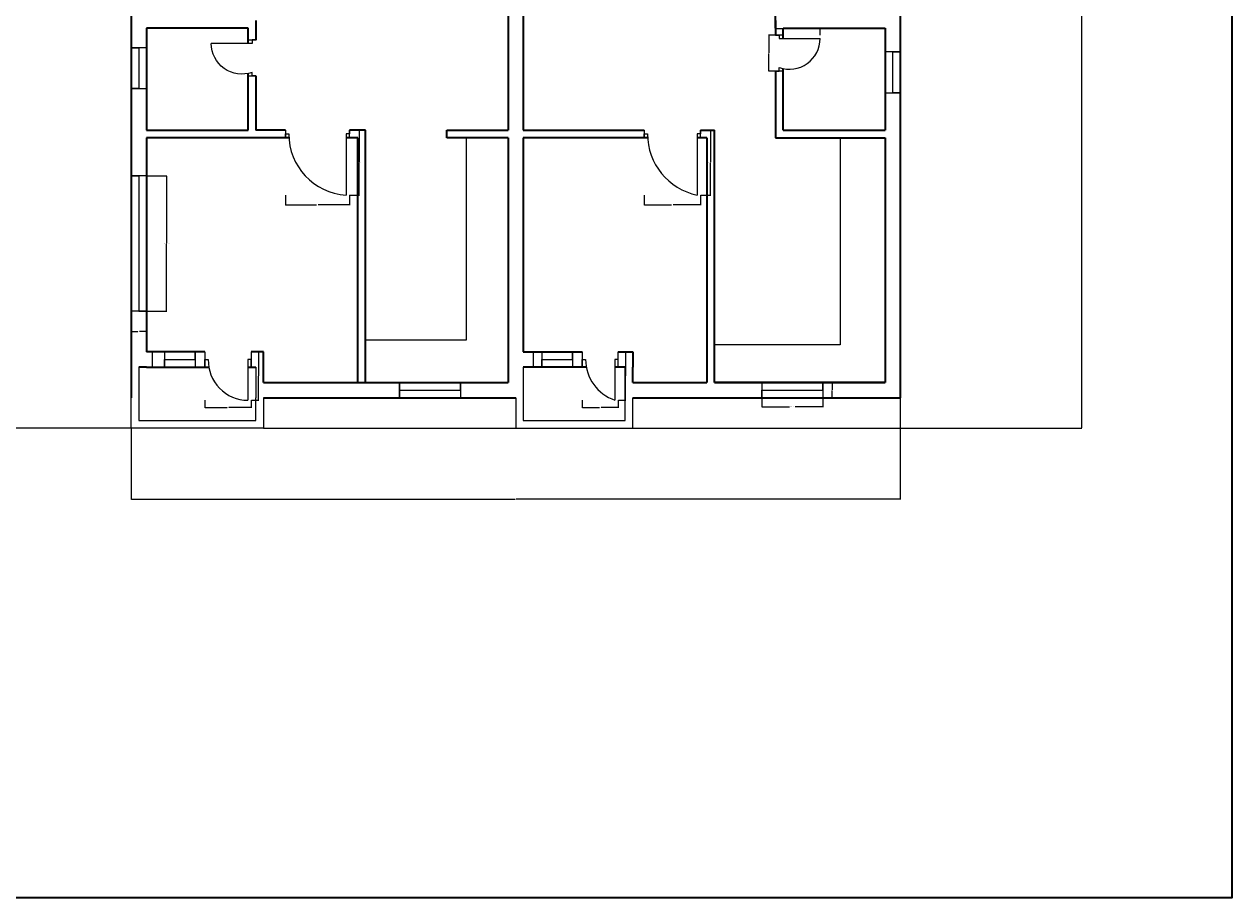
# Model space of a CAD drawing. Units: inches. Extents: x 2250 to 3629, y 982 to 2740.
# Tile 6 of 12: x 2918 to 3629, y 982 to 1497. Entities that reach past the tile are written whole.
import ezdxf

# ---------------------------------------------------------------- set-up
doc = ezdxf.new("R2010")
doc.units = ezdxf.units.IN
for name, color, linetype, lineweight in [('A-ANNO-DIMS', 2, 'Continuous', 18), ('A-ANNO-TTLB', 7, 'Continuous', 35), ('A-DOOR', 3, 'Continuous', 18), ('A-FLOR-DECK', 7, 'Continuous', 25), ('A-FLOR-FIXT', 9, 'Continuous', 18), ('A-GLAZ', 4, 'Continuous', 18), ('A-WALL', 7, 'Continuous', 35)]:
    doc.layers.add(name, color=color, linetype=linetype, lineweight=lineweight)
doc.styles.get("Standard").update_dxf_attribs({"font": 'arial.ttf'})
doc.dimstyles.get("Standard").update_dxf_attribs({"dimtxt": 0.18, "dimasz": 0.18, "dimexe": 0.18, "dimexo": 0.0625, "dimgap": 0.09, "dimtad": 0, "dimtih": 1, "dimtoh": 1, "dimdec": 4, "dimzin": 0, "dimdsep": 46, "dimtxsty": 'Standard', "dimcen": 0.09, "dimadec": 0, "dimazin": 0, "dimtfac": 1, "dimtdec": 4, "dimtofl": 0, "dimtmove": 0, "dimatfit": 3, "dimfxl": 1, "dimtolj": 1, "dimtzin": 0, "dimarcsym": 0})

# ---------------------------------------------------------------- blocks, each defined once
blk = doc.blocks.new('DR-24-BATH-SE')
for p, q in [((4.5, 21.1), (0, 21.1)), ((0, 21.1), (2.25, 21.1)), ((2.25, 21.1), (2.25, 19.1)), ((2.25, 19.1), (26.25, 19.1)), ((4.5, 0), (0, 0)), ((0, 0), (2.25, 0)), ((2.25, 0), (2.25, 2))]:
    blk.add_line(p, q)
blk.add_arc((8.16, 19.1), 18.09, 250.94149, 0)
blk = doc.blocks.new('DR-36-BED-SW')
for p, q in [((0, 38.25), (0, 33.75)), ((0, 33.75), (0, 36)), ((0, 36), (2, 36)), ((37.72, 36), (35.72, 36)), ((35.72, 36), (35.72, 0)), ((37.72, 33.75), (37.72, 38.25)), ((37.72, 38.25), (37.72, 36))]:
    blk.add_line(p, q)
blk.add_arc((38.08, 36), 36.08, 180, 266.25862)
blk = doc.blocks.new('DR-36-BED-SE')
for p, q in [((0, 38.25), (0, 33.75)), ((0, 33.75), (0, 36)), ((0, 36), (2, 36)), ((33.26, 36), (31.26, 36)), ((31.26, 36), (31.26, 0)), ((33.26, 33.75), (33.26, 38.25)), ((33.26, 38.25), (33.26, 36))]:
    blk.add_line(p, q)
blk.add_arc((38.78, 36), 36.78, 180, 258.21311)
blk = doc.blocks.new('DR-24-DECK-SW')
for p, q in [((0, 28.5), (0, 19.5)), ((27.27, 28.5), (27.27, 19.5)), ((0, 19.5), (0, 24)), ((0, 24), (2, 24)), ((27.27, 24), (25.27, 24)), ((25.27, 24), (25.27, 0)), ((27.27, 19.5), (27.27, 24))]:
    blk.add_line(p, q)
blk.add_arc((25.27, 23.29), 23.29, 178.24083, 270)
blk = doc.blocks.new('DR-24-DECK-SE')
for p, q in [((0, 28.5), (0, 19.5)), ((21.23, 19.5), (21.23, 28.5)), ((0, 19.5), (0, 24)), ((0, 24), (2, 24)), ((21.23, 24), (19.23, 24)), ((19.23, 24), (19.23, 0))]:
    blk.add_line(p, q)
blk.add_arc((27.33, 24), 25.33, 180, 251.36498)
blk = doc.blocks.new('WIN-24-DECK-NE')
for p, q in [((0, 4.5), (0, 9)), ((0, 9), (0, 0)), ((24, 0), (24, 9)), ((24, 9), (24, 4.5)), ((24, 4.5), (0, 4.5))]:
    blk.add_line(p, q)
blk = doc.blocks.new('WIN-36-KITCHEN-NE')
for p, q in [((0, 9), (0, 0)), ((0, 0), (0, 9)), ((0, 9), (0, 4.5)), ((36, 4.5), (36, 9)), ((36, 9), (36, 0)), ((0, 4.5), (36, 4.5))]:
    blk.add_line(p, q)
blk = doc.blocks.new('WIN-18-DECK-SW')
for p, q in [((0, 9), (0, 0)), ((18.04, 4.5), (18.04, 9)), ((18.04, 9), (18.04, 0)), ((0, 0), (0, 4.5)), ((0, 4.5), (18.04, 4.5))]:
    blk.add_line(p, q)
blk = doc.blocks.new('WIN-36-KITCHEN-SE')
for p, q in [((0, 9), (0, 0)), ((36, 4.5), (36, 9)), ((36, 9), (36, 0)), ((0, 0), (0, 4.5)), ((0, 4.5), (36, 4.5))]:
    blk.add_line(p, q)
blk = doc.blocks.new('WIN-BED-SW')
for p, q in [((9, 79.76), (0, 79.76)), ((0, 79.76), (4.5, 79.76)), ((4.5, 79.76), (4.5, 0)), ((9, 0), (0, 0)), ((4.5, 0), (9, 0))]:
    blk.add_line(p, q)
blk = doc.blocks.new('*D91')
at = {"layer": 'A-ANNO-DIMS', "color": 0, "lineweight": -2, "transparency": 16777216}
for p, q in [((3352.67, 1276.67), (3352.67, 1271.16)), ((3388.67, 1276.67), (3388.67, 1271.16)), ((3352.85, 1271.34), (3368.97, 1271.34)), ((3388.49, 1271.34), (3372.37, 1271.34))]:
    blk.add_line(p, q, dxfattribs=at)
at = {"layer": 'A-ANNO-DIMS', "color": 0, "transparency": 16777216}
for points in [[(3352.85, 1271.37), (3352.85, 1271.31), (3352.67, 1271.34)], [(3388.49, 1271.37), (3388.49, 1271.31), (3388.67, 1271.34)]]:
    blk.add_solid(points, dxfattribs=at)
at = {"layer": 'Defpoints', "color": 0, "transparency": 16777216}
for p in [(3352.67, 1276.74), (3388.67, 1276.74), (3388.67, 1271.34)]:
    blk.add_point(p, dxfattribs=at)
at = {"layer": 'A-ANNO-DIMS', "color": 0, "transparency": 16777216, "insert": (3370.67, 1271.34), "char_height": 0.18, "attachment_point": 5}
blk.add_mtext('\\A1;KITCHEN WINDOW 36 TYP.', dxfattribs=at)
blk = doc.blocks.new('*D92')
at = {"layer": 'A-ANNO-DIMS', "color": 0, "lineweight": -2, "transparency": 16777216}
for p, q in [((3388.73, 1285.74), (3394.25, 1285.74)), ((3394.07, 1285.56), (3394.07, 1281.42)), ((3394.07, 1276.92), (3394.07, 1281.05)), ((3388.73, 1276.74), (3394.25, 1276.74))]:
    blk.add_line(p, q, dxfattribs=at)
at = {"layer": 'A-ANNO-DIMS', "color": 0, "transparency": 16777216}
for points in [[(3394.04, 1285.56), (3394.1, 1285.56), (3394.07, 1285.74)], [(3394.04, 1276.92), (3394.1, 1276.92), (3394.07, 1276.74)]]:
    blk.add_solid(points, dxfattribs=at)
at = {"layer": 'Defpoints', "color": 0, "transparency": 16777216}
for p in [(3388.67, 1285.74), (3394.07, 1285.74), (3388.67, 1276.74)]:
    blk.add_point(p, dxfattribs=at)
at = {"layer": 'A-ANNO-DIMS', "color": 0, "transparency": 16777216, "insert": (3394.07, 1281.24), "char_height": 0.18, "attachment_point": 5}
blk.add_mtext('\\A1;9 TYP.', dxfattribs=at)
blk = doc.blocks.new('*D93')
at = {"layer": 'A-ANNO-DIMS', "color": 0, "lineweight": -2, "transparency": 16777216}
for p, q in [((2990.29, 1407.36), (3002.37, 1407.36)), ((3002.19, 1407.18), (3002.19, 1367.66)), ((3002.19, 1327.77), (3002.19, 1367.29)), ((2990.29, 1327.59), (3002.37, 1327.59))]:
    blk.add_line(p, q, dxfattribs=at)
at = {"layer": 'A-ANNO-DIMS', "color": 0, "transparency": 16777216}
for points in [[(3002.16, 1407.18), (3002.22, 1407.18), (3002.19, 1407.36)], [(3002.16, 1327.77), (3002.22, 1327.77), (3002.19, 1327.59)]]:
    blk.add_solid(points, dxfattribs=at)
at = {"layer": 'Defpoints', "color": 0, "transparency": 16777216}
for p in [(2990.23, 1407.36), (3002.19, 1407.36), (2990.23, 1327.59)]:
    blk.add_point(p, dxfattribs=at)
at = {"layer": 'A-ANNO-DIMS', "color": 0, "transparency": 16777216, "insert": (3002.19, 1367.47), "char_height": 0.18, "attachment_point": 5}
blk.add_mtext('\\A1;BEDROOM WINDOW 80 TYP.', dxfattribs=at)
blk = doc.blocks.new('*D94')
at = {"layer": 'A-ANNO-DIMS', "color": 0, "lineweight": -2, "transparency": 16777216}
for p, q in [((2981.23, 1327.53), (2981.23, 1315.45)), ((2990.23, 1327.53), (2990.23, 1315.45)), ((2981.41, 1315.63), (2985.27, 1315.63)), ((2990.05, 1315.63), (2986.18, 1315.63))]:
    blk.add_line(p, q, dxfattribs=at)
at = {"layer": 'A-ANNO-DIMS', "color": 0, "transparency": 16777216}
for points in [[(2981.41, 1315.66), (2981.41, 1315.6), (2981.23, 1315.63)], [(2990.05, 1315.66), (2990.05, 1315.6), (2990.23, 1315.63)]]:
    blk.add_solid(points, dxfattribs=at)
at = {"layer": 'Defpoints', "color": 0, "transparency": 16777216}
for p in [(2981.23, 1327.59), (2990.23, 1327.59), (2990.23, 1315.63)]:
    blk.add_point(p, dxfattribs=at)
at = {"layer": 'A-ANNO-DIMS', "color": 0, "transparency": 16777216, "insert": (2985.73, 1315.63), "char_height": 0.18, "attachment_point": 5}
blk.add_mtext('\\A1;9 TYP.', dxfattribs=at)
blk = doc.blocks.new('*D97')
at = {"layer": 'A-ANNO-DIMS', "color": 0, "lineweight": -2, "transparency": 16777216}
for p, q in [((3360.73, 1490.19), (3360.73, 1494.24)), ((3360.91, 1494.06), (3372.55, 1494.06)), ((3386.8, 1494.06), (3375.16, 1494.06)), ((3386.98, 1490.19), (3386.98, 1494.24))]:
    blk.add_line(p, q, dxfattribs=at)
at = {"layer": 'A-ANNO-DIMS', "color": 0, "transparency": 16777216}
for points in [[(3360.91, 1494.09), (3360.91, 1494.03), (3360.73, 1494.06)], [(3386.8, 1494.09), (3386.8, 1494.03), (3386.98, 1494.06)]]:
    blk.add_solid(points, dxfattribs=at)
at = {"layer": 'Defpoints', "color": 0, "transparency": 16777216}
for p in [(3386.98, 1494.06), (3360.73, 1490.12), (3386.98, 1490.12)]:
    blk.add_point(p, dxfattribs=at)
at = {"layer": 'A-ANNO-DIMS', "color": 0, "transparency": 16777216, "insert": (3373.85, 1494.06), "char_height": 0.18, "attachment_point": 5}
blk.add_mtext('\\A1;BATH DOOR 26 TYP.', dxfattribs=at)
blk = doc.blocks.new('*D98')
at = {"layer": 'A-ANNO-DIMS', "color": 0, "lineweight": -2, "transparency": 16777216}
for p, q in [((3360.66, 1490.12), (3356.61, 1490.12)), ((3356.79, 1489.94), (3356.79, 1479.75)), ((3356.79, 1469.2), (3356.79, 1479.39)), ((3360.66, 1469.02), (3356.61, 1469.02))]:
    blk.add_line(p, q, dxfattribs=at)
at = {"layer": 'A-ANNO-DIMS', "color": 0, "transparency": 16777216}
for points in [[(3356.76, 1489.94), (3356.82, 1489.94), (3356.79, 1490.12)], [(3356.76, 1469.2), (3356.82, 1469.2), (3356.79, 1469.02)]]:
    blk.add_solid(points, dxfattribs=at)
at = {"layer": 'Defpoints', "color": 0, "transparency": 16777216}
for p in [(3356.79, 1490.12), (3360.73, 1490.12), (3360.73, 1469.02)]:
    blk.add_point(p, dxfattribs=at)
at = {"layer": 'A-ANNO-DIMS', "color": 0, "transparency": 16777216, "insert": (3356.79, 1479.57), "char_height": 0.18, "attachment_point": 5}
blk.add_mtext('\\A1;21 TYP.', dxfattribs=at)
blk = doc.blocks.new('*D121')
at = {"layer": 'A-ANNO-DIMS', "color": 0, "lineweight": -2, "transparency": 16777216}
for p, q in [((3109.88, 1434.24), (3115.73, 1434.24)), ((3115.55, 1434.06), (3115.55, 1415.29)), ((3115.55, 1396.17), (3115.55, 1414.93)), ((3109.88, 1395.99), (3115.73, 1395.99))]:
    blk.add_line(p, q, dxfattribs=at)
at = {"layer": 'A-ANNO-DIMS', "color": 0, "transparency": 16777216}
for points in [[(3115.52, 1434.06), (3115.58, 1434.06), (3115.55, 1434.24)], [(3115.52, 1396.17), (3115.58, 1396.17), (3115.55, 1395.99)]]:
    blk.add_solid(points, dxfattribs=at)
at = {"layer": 'Defpoints', "color": 0, "transparency": 16777216}
for p in [(3109.81, 1434.24), (3115.55, 1434.24), (3109.81, 1395.99)]:
    blk.add_point(p, dxfattribs=at)
at = {"layer": 'A-ANNO-DIMS', "color": 0, "transparency": 16777216, "insert": (3115.55, 1415.11), "char_height": 0.18, "attachment_point": 5}
blk.add_mtext('\\A1;BEDROOM DOOR 38 TYP.', dxfattribs=at)
blk = doc.blocks.new('*D122')
at = {"layer": 'A-ANNO-DIMS', "color": 0, "lineweight": -2, "transparency": 16777216}
for p, q in [((3072.09, 1395.92), (3072.09, 1390.07)), ((3109.81, 1395.92), (3109.81, 1390.07)), ((3072.27, 1390.25), (3090.42, 1390.25)), ((3109.63, 1390.25), (3091.48, 1390.25))]:
    blk.add_line(p, q, dxfattribs=at)
at = {"layer": 'A-ANNO-DIMS', "color": 0, "transparency": 16777216}
for points in [[(3072.27, 1390.28), (3072.27, 1390.22), (3072.09, 1390.25)], [(3109.63, 1390.28), (3109.63, 1390.22), (3109.81, 1390.25)]]:
    blk.add_solid(points, dxfattribs=at)
at = {"layer": 'Defpoints', "color": 0, "transparency": 16777216}
for p in [(3072.09, 1395.99), (3109.81, 1395.99), (3109.81, 1390.25)]:
    blk.add_point(p, dxfattribs=at)
at = {"layer": 'A-ANNO-DIMS', "color": 0, "transparency": 16777216, "insert": (3090.95, 1390.25), "char_height": 0.18, "attachment_point": 5}
blk.add_mtext('\\A1;38 TYP.', dxfattribs=at)
blk = doc.blocks.new('*D123')
at = {"layer": 'A-ANNO-DIMS', "color": 0, "lineweight": -2, "transparency": 16777216}
for p, q in [((3316.69, 1434.24), (3322.55, 1434.24)), ((3322.37, 1434.06), (3322.37, 1415.29)), ((3322.37, 1396.17), (3322.37, 1414.93)), ((3316.69, 1395.99), (3322.55, 1395.99))]:
    blk.add_line(p, q, dxfattribs=at)
at = {"layer": 'A-ANNO-DIMS', "color": 0, "transparency": 16777216}
for points in [[(3322.34, 1434.06), (3322.4, 1434.06), (3322.37, 1434.24)], [(3322.34, 1396.17), (3322.4, 1396.17), (3322.37, 1395.99)]]:
    blk.add_solid(points, dxfattribs=at)
at = {"layer": 'Defpoints', "color": 0, "transparency": 16777216}
for p in [(3316.63, 1434.24), (3322.37, 1434.24), (3316.63, 1395.99)]:
    blk.add_point(p, dxfattribs=at)
at = {"layer": 'A-ANNO-DIMS', "color": 0, "transparency": 16777216, "insert": (3322.37, 1415.11), "char_height": 0.18, "attachment_point": 5}
blk.add_mtext('\\A1;BEDROOM DOOR 38 TYP.', dxfattribs=at)
blk = doc.blocks.new('*D124')
at = {"layer": 'A-ANNO-DIMS', "color": 0, "lineweight": -2, "transparency": 16777216}
for p, q in [((3283.37, 1395.92), (3283.37, 1390.07)), ((3316.63, 1395.92), (3316.63, 1390.07)), ((3283.55, 1390.25), (3299.47, 1390.25)), ((3316.45, 1390.25), (3300.53, 1390.25))]:
    blk.add_line(p, q, dxfattribs=at)
at = {"layer": 'A-ANNO-DIMS', "color": 0, "transparency": 16777216}
for points in [[(3283.55, 1390.28), (3283.55, 1390.22), (3283.37, 1390.25)], [(3316.45, 1390.28), (3316.45, 1390.22), (3316.63, 1390.25)]]:
    blk.add_solid(points, dxfattribs=at)
at = {"layer": 'Defpoints', "color": 0, "transparency": 16777216}
for p in [(3283.37, 1395.99), (3316.63, 1395.99), (3316.63, 1390.25)]:
    blk.add_point(p, dxfattribs=at)
at = {"layer": 'A-ANNO-DIMS', "color": 0, "transparency": 16777216, "insert": (3300, 1390.25), "char_height": 0.18, "attachment_point": 5}
blk.add_mtext('\\A1;33 TYP.', dxfattribs=at)
blk = doc.blocks.new('*D141')
at = {"layer": 'A-ANNO-DIMS', "color": 0, "lineweight": -2, "transparency": 16777216}
for p, q in [((3052.06, 1303.74), (3056.46, 1303.74)), ((3056.28, 1303.56), (3056.28, 1289.67)), ((3056.28, 1275.42), (3056.28, 1289.3)), ((3052.06, 1275.24), (3056.46, 1275.24))]:
    blk.add_line(p, q, dxfattribs=at)
at = {"layer": 'A-ANNO-DIMS', "color": 0, "transparency": 16777216}
for points in [[(3056.25, 1303.56), (3056.31, 1303.56), (3056.28, 1303.74)], [(3056.25, 1275.42), (3056.31, 1275.42), (3056.28, 1275.24)]]:
    blk.add_solid(points, dxfattribs=at)
at = {"layer": 'Defpoints', "color": 0, "transparency": 16777216}
for p in [(3052, 1303.74), (3056.28, 1303.74), (3052, 1275.24)]:
    blk.add_point(p, dxfattribs=at)
at = {"layer": 'A-ANNO-DIMS', "color": 0, "transparency": 16777216, "insert": (3056.28, 1289.49), "char_height": 0.18, "attachment_point": 5}
blk.add_mtext('\\A1;DECK DOOR 29 TYP.', dxfattribs=at)
blk = doc.blocks.new('*D142')
at = {"layer": 'A-ANNO-DIMS', "color": 0, "lineweight": -2, "transparency": 16777216}
for p, q in [((3024.73, 1275.17), (3024.73, 1270.78)), ((3052, 1275.17), (3052, 1270.78)), ((3024.91, 1270.96), (3037.83, 1270.96)), ((3051.82, 1270.96), (3038.89, 1270.96))]:
    blk.add_line(p, q, dxfattribs=at)
at = {"layer": 'A-ANNO-DIMS', "color": 0, "transparency": 16777216}
for points in [[(3024.91, 1270.99), (3024.91, 1270.93), (3024.73, 1270.96)], [(3051.82, 1270.99), (3051.82, 1270.93), (3052, 1270.96)]]:
    blk.add_solid(points, dxfattribs=at)
at = {"layer": 'Defpoints', "color": 0, "transparency": 16777216}
for p in [(3024.73, 1275.24), (3052, 1275.24), (3052, 1270.96)]:
    blk.add_point(p, dxfattribs=at)
at = {"layer": 'A-ANNO-DIMS', "color": 0, "transparency": 16777216, "insert": (3038.36, 1270.96), "char_height": 0.18, "attachment_point": 5}
blk.add_mtext('\\A1;27 TYP.', dxfattribs=at)
blk = doc.blocks.new('*D143')
at = {"layer": 'A-ANNO-DIMS', "color": 0, "lineweight": -2, "transparency": 16777216}
for p, q in [((3268.22, 1303.74), (3272.62, 1303.74)), ((3272.44, 1303.56), (3272.44, 1289.67)), ((3272.44, 1275.42), (3272.44, 1289.3)), ((3268.22, 1275.24), (3272.62, 1275.24))]:
    blk.add_line(p, q, dxfattribs=at)
at = {"layer": 'A-ANNO-DIMS', "color": 0, "transparency": 16777216}
for points in [[(3272.41, 1303.56), (3272.47, 1303.56), (3272.44, 1303.74)], [(3272.41, 1275.42), (3272.47, 1275.42), (3272.44, 1275.24)]]:
    blk.add_solid(points, dxfattribs=at)
at = {"layer": 'Defpoints', "color": 0, "transparency": 16777216}
for p in [(3268.16, 1303.74), (3272.44, 1303.74), (3268.16, 1275.24)]:
    blk.add_point(p, dxfattribs=at)
at = {"layer": 'A-ANNO-DIMS', "color": 0, "transparency": 16777216, "insert": (3272.44, 1289.49), "char_height": 0.18, "attachment_point": 5}
blk.add_mtext('\\A1;DECK DOOR 29 TYP.', dxfattribs=at)
blk = doc.blocks.new('*D144')
at = {"layer": 'A-ANNO-DIMS', "color": 0, "lineweight": -2, "transparency": 16777216}
for p, q in [((3246.93, 1275.17), (3246.93, 1270.78)), ((3268.16, 1275.17), (3268.16, 1270.78)), ((3247.11, 1270.96), (3257.02, 1270.96)), ((3267.98, 1270.96), (3258.07, 1270.96))]:
    blk.add_line(p, q, dxfattribs=at)
at = {"layer": 'A-ANNO-DIMS', "color": 0, "transparency": 16777216}
for points in [[(3247.11, 1270.99), (3247.11, 1270.93), (3246.93, 1270.96)], [(3267.98, 1270.99), (3267.98, 1270.93), (3268.16, 1270.96)]]:
    blk.add_solid(points, dxfattribs=at)
at = {"layer": 'Defpoints', "color": 0, "transparency": 16777216}
for p in [(3246.93, 1275.24), (3268.16, 1275.24), (3268.16, 1270.96)]:
    blk.add_point(p, dxfattribs=at)
at = {"layer": 'A-ANNO-DIMS', "color": 0, "transparency": 16777216, "insert": (3257.54, 1270.96), "char_height": 0.18, "attachment_point": 5}
blk.add_mtext('\\A1;21 TYP.', dxfattribs=at)
blk = doc.blocks.new('*D171')
at = {"layer": 'A-ANNO-DIMS', "color": 0, "lineweight": -2, "transparency": 16777216}
for p, q in [((3434.23, 1276.67), (3434.23, 1216.81)), ((2981.23, 1258.67), (2981.23, 1216.81)), ((2981.41, 1216.99), (3207.43, 1216.99)), ((3434.05, 1216.99), (3208.02, 1216.99))]:
    blk.add_line(p, q, dxfattribs=at)
at = {"layer": 'A-ANNO-DIMS', "color": 0, "transparency": 16777216}
for points in [[(2981.41, 1217.02), (2981.41, 1216.96), (2981.23, 1216.99)], [(3434.05, 1217.02), (3434.05, 1216.96), (3434.23, 1216.99)]]:
    blk.add_solid(points, dxfattribs=at)
at = {"layer": 'Defpoints', "color": 0, "transparency": 16777216}
for p in [(3434.23, 1276.74), (2981.23, 1258.74), (3434.23, 1216.99)]:
    blk.add_point(p, dxfattribs=at)
at = {"layer": 'A-ANNO-DIMS', "color": 0, "transparency": 16777216, "insert": (3207.73, 1216.99), "char_height": 0.18, "attachment_point": 5}
blk.add_mtext('\\A1;453', dxfattribs=at)
blk = doc.blocks.new('*D172')
at = {"layer": 'A-ANNO-DIMS', "color": 0, "lineweight": -2, "transparency": 16777216}
for p, q in [((3433.02, 2070.24), (3541.21, 2070.24)), ((3541.03, 2070.06), (3541.03, 1664.67)), ((3541.03, 1258.92), (3541.03, 1664.3)), ((3059.29, 1258.74), (3541.21, 1258.74))]:
    blk.add_line(p, q, dxfattribs=at)
at = {"layer": 'A-ANNO-DIMS', "color": 0, "transparency": 16777216}
for points in [[(3541, 2070.06), (3541.06, 2070.06), (3541.03, 2070.24)], [(3541, 1258.92), (3541.06, 1258.92), (3541.03, 1258.74)]]:
    blk.add_solid(points, dxfattribs=at)
at = {"layer": 'Defpoints', "color": 0, "transparency": 16777216}
for p in [(3432.96, 2070.24), (3541.03, 2070.24), (3059.23, 1258.74)]:
    blk.add_point(p, dxfattribs=at)
at = {"layer": 'A-ANNO-DIMS', "color": 0, "transparency": 16777216, "insert": (3541.03, 1664.49), "char_height": 0.18, "attachment_point": 5}
blk.add_mtext('\\A1;811.5', dxfattribs=at)
blk = doc.blocks.new('*D173')
at = {"layer": 'A-ANNO-DIMS', "color": 0, "lineweight": -2, "transparency": 16777216}
for p, q in [((2932.01, 1947.92), (2890.14, 1947.92)), ((2890.32, 1947.74), (2890.32, 1603.51)), ((2890.32, 1258.92), (2890.32, 1603.15)), ((2981.16, 1258.74), (2890.14, 1258.74))]:
    blk.add_line(p, q, dxfattribs=at)
at = {"layer": 'A-ANNO-DIMS', "color": 0, "transparency": 16777216}
for points in [[(2890.29, 1947.74), (2890.35, 1947.74), (2890.32, 1947.92)], [(2890.29, 1258.92), (2890.35, 1258.92), (2890.32, 1258.74)]]:
    blk.add_solid(points, dxfattribs=at)
at = {"layer": 'Defpoints', "color": 0, "transparency": 16777216}
for p in [(2932.07, 1947.92), (2890.32, 1258.74), (2981.23, 1258.74)]:
    blk.add_point(p, dxfattribs=at)
at = {"layer": 'A-ANNO-DIMS', "color": 0, "transparency": 16777216, "insert": (2890.32, 1603.33), "char_height": 0.18, "attachment_point": 5}
blk.add_mtext('\\A1;689.2', dxfattribs=at)

msp = doc.modelspace()

# ---------------------------------------------------------------- linework, layer by layer
at = {"layer": 'A-ANNO-TTLB'}
msp.add_lwpolyline([(2249.6849, 2739.593), (3629.4532, 2739.593), (3629.4532, 982.3108), (2249.6849, 982.3108)], close=True, dxfattribs=at)
at = {"layer": 'A-FLOR-DECK'}
for p, q in [((2985.7267, 1294.7354), (2985.7267, 1263.2354)), ((3054.7267, 1294.7354), (3054.7267, 1276.7354)), ((3212.2267, 1294.7354), (3212.2267, 1276.7354)), ((3272.2453, 1263.2354), (3272.2453, 1294.7354)), ((2981.2267, 1258.7354), (2981.2267, 1276.7354)), ((3054.7267, 1263.2354), (3054.7267, 1276.7354)), ((3059.2267, 1276.7354), (3059.2267, 1258.7354)), ((3207.7267, 1276.7354), (3207.7267, 1258.7354)), ((3212.2267, 1276.7354), (3212.2267, 1263.2354)), ((3276.7453, 1258.7354), (3276.7453, 1276.7354)), ((2985.7267, 1263.2354), (3054.7267, 1263.2354)), ((3212.2267, 1263.2354), (3272.2453, 1263.2354)), ((3059.2267, 1258.7354), (2981.2267, 1258.7354)), ((3207.7267, 1258.7354), (3276.7453, 1258.7354))]:
    msp.add_line(p, q, dxfattribs=at)
at = {"layer": 'A-FLOR-FIXT'}
for p, q in [((3178.6142, 1429.7354), (3178.6142, 1310.6354)), ((3398.8991, 1429.7354), (3398.8991, 1307.7437)), ((3178.6142, 1310.6354), (3119.2267, 1310.6354)), ((3398.8991, 1307.7437), (3324.7267, 1307.7437))]:
    msp.add_line(p, q, dxfattribs=at)
at = {"layer": 'A-GLAZ'}
for p, q in [((2993.6065, 1303.7354), (2993.6065, 1294.7354)), ((3218.0295, 1303.7354), (3218.0295, 1296.6878)), ((3218.0295, 1296.6878), (3218.0295, 1294.7354))]:
    msp.add_line(p, q, dxfattribs=at)
at = {"layer": 'A-WALL'}
for p, q in [((2981.2267, 2047.7354), (2981.2267, 1276.7354)), ((3434.2267, 2029.7354), (3434.2267, 1276.7354)), ((3203.2267, 1638.2354), (3203.2267, 1434.2354)), ((3212.2267, 1638.2354), (3212.2267, 1434.2354)), ((3360.7267, 1494.2354), (3360.7267, 1506.4808)), ((2990.2267, 1494.2354), (2990.2267, 1434.2354)), ((3050.2267, 1494.2354), (2990.2267, 1494.2354)), ((3050.2267, 1485.263), (3050.2267, 1494.2354)), ((3054.7267, 1498.7354), (3054.7267, 1487.263)), ((3360.7267, 1498.7354), (3360.7267, 1494.2354)), ((3360.7267, 1494.2354), (3360.7267, 1490.123)), ((3365.2267, 1494.2354), (3425.2267, 1494.2354)), ((3365.2267, 1488.123), (3365.2267, 1494.2354)), ((3425.2267, 1494.2354), (3425.2267, 1434.2354)), ((3050.2267, 1434.2354), (3050.2267, 1467.5923)), ((3054.7267, 1466.2174), (3054.7267, 1434.2354)), ((3360.7267, 1469.0225), (3360.7267, 1429.7354)), ((3365.2267, 1434.2354), (3365.2267, 1470.4043)), ((2990.2267, 1434.2354), (3050.2267, 1434.2354)), ((2990.2267, 1429.7354), (2990.2267, 1303.7354)), ((3074.1608, 1429.7354), (2990.2267, 1429.7354)), ((3072.0906, 1434.2354), (3054.7267, 1434.2354)), ((3114.7267, 1429.7354), (3107.8133, 1429.7354)), ((3119.2267, 1434.2354), (3109.8133, 1434.2354)), ((3114.7267, 1405.7354), (3114.7267, 1429.7354)), ((3119.2267, 1285.7354), (3119.2267, 1434.2354)), ((3167.2441, 1434.2354), (3203.2267, 1434.2354)), ((3167.2441, 1429.7354), (3167.2441, 1434.2354)), ((3203.2267, 1429.7354), (3167.2441, 1429.7354)), ((3203.2267, 1429.7354), (3203.2267, 1285.7354)), ((3212.2267, 1434.2354), (3283.3663, 1434.2354)), ((3212.2267, 1429.7354), (3212.2267, 1303.7354)), ((3285.4352, 1429.7354), (3212.2267, 1429.7354)), ((3320.2267, 1429.7354), (3314.6295, 1429.7354)), ((3316.6295, 1434.2354), (3324.7267, 1434.2354)), ((3320.2267, 1429.7354), (3320.2267, 1285.7354)), ((3324.7267, 1429.7354), (3324.7267, 1434.2354)), ((3324.7267, 1285.7354), (3324.7267, 1429.7354)), ((3360.7267, 1429.7354), (3425.2267, 1429.7354)), ((3360.7267, 1429.7354), (3365.2267, 1429.7354)), ((3365.2267, 1434.2354), (3425.2267, 1434.2354)), ((3425.2267, 1429.7354), (3425.2267, 1285.7354)), ((3114.7267, 1285.7354), (3114.7267, 1405.7354)), ((3024.7267, 1303.7354), (2990.2267, 1303.7354)), ((3059.2267, 1303.7354), (3052.0009, 1303.7354)), ((3059.2267, 1285.7354), (3059.2267, 1303.7354)), ((3212.2267, 1303.7354), (3246.9277, 1303.7354)), ((3268.1623, 1303.7354), (3276.7453, 1303.7354)), ((3276.7453, 1303.7354), (3276.7453, 1294.7354)), ((2990.2267, 1294.7354), (2985.7267, 1294.7354)), ((2990.2267, 1294.7354), (3027.0255, 1294.7354)), ((3050.0009, 1294.7354), (3054.7267, 1294.7354)), ((3249.3306, 1294.7354), (3212.2267, 1294.7354)), ((3272.2453, 1294.7354), (3266.1623, 1294.7354)), ((3276.7453, 1285.7354), (3276.7453, 1294.7354)), ((3059.2267, 1285.7354), (3203.2267, 1285.7354)), ((3059.2267, 1285.7354), (3114.7267, 1285.7354)), ((3114.7267, 1285.7354), (3119.2267, 1285.7354)), ((3276.7453, 1285.7354), (3320.2267, 1285.7354)), ((3324.7267, 1285.7354), (3425.2267, 1285.7354)), ((3425.2267, 1285.7354), (3324.7267, 1285.7354)), ((3059.2267, 1276.7354), (3207.7267, 1276.7354)), ((3276.7453, 1276.7354), (3434.2267, 1276.7354))]:
    msp.add_line(p, q, dxfattribs=at)

# ---------------------------------------------------------------- block references
at = {"layer": 'A-DOOR', "extrusion": (0, 0, -1), "zscale": -1, "rotation": 359.9465721628409}
msp.add_blockref('DR-24-BATH-SE', (-3054.7359, 1466.1894), dxfattribs=at)
at = {"layer": 'A-DOOR'}
for name, p in [('DR-24-BATH-SE', (3360.7265, 1469.022)), ('DR-36-BED-SW', (3072.0905, 1395.985)), ('DR-36-BED-SE', (3283.3665, 1395.985)), ('DR-24-DECK-SW', (3024.7265, 1275.235)), ('DR-24-DECK-SE', (3246.9275, 1275.235))]:
    msp.add_blockref(name, p, dxfattribs=at)
at = {"layer": 'A-GLAZ'}
for name, p, rotation in [('WIN-24-DECK-NE', (2990.2272, 1458.7153), 90.0000000000019), ('WIN-24-DECK-NE', (3425.2263, 1480.2354), 269.9999999999954), ('WIN-18-DECK-SW', (3223.0919, 1294.7087), 0.1672301246917131)]:
    msp.add_blockref(name, p, dxfattribs=dict(at, rotation=rotation))
for name, p in [('WIN-BED-SW', (2981.2265, 1327.592)), ('WIN-18-DECK-SW', (3000.9015, 1294.735)), ('WIN-36-KITCHEN-NE', (3139.3089, 1276.735)), ('WIN-36-KITCHEN-SE', (3352.6695, 1276.735))]:
    msp.add_blockref(name, p, dxfattribs=at)

# ---------------------------------------------------------------- dimensions: what is measured, and where the dimension line sits
at = {"layer": 'A-ANNO-DIMS'}
for base, p1, p2, picture, middle in [((3541.0278, 2070.2354), (3059.2267, 1258.7354), (3432.9579, 2070.2354), '*D172', (3541.0278, 1664.4854)), ((2890.3241, 1258.7354), (2932.0741, 1947.9231), (2981.2267, 1258.7354), '*D173', (2890.3241, 1603.3293))]:
    dim = msp.add_linear_dim(base=base, p1=p1, p2=p2, angle=90, dimstyle='Standard', override={"dimdec": 1, "dimlfac": 1, "dimrnd": 0, "dimzin": 0, "dimdsep": 46, "dimlunit": 2}, dxfattribs=at)
    dim.commit()
    dim.dimension.update_dxf_attribs({"geometry": picture, "text_midpoint": middle})
for base, p1, p2, text, picture, middle in [((3386.9767, 1494.0605), (3360.7267, 1490.123), (3386.9767, 1490.123), 'BATH DOOR <> TYP.', '*D97', (3373.8517, 1494.0605)), ((3109.8133, 1390.2479), (3072.0906, 1395.9854), (3109.8133, 1395.9854), '<> TYP.', '*D122', (3090.952, 1390.2479)), ((3316.6295, 1390.2479), (3283.3663, 1395.9854), (3316.6295, 1395.9854), '<> TYP.', '*D124', (3299.9979, 1390.2479)), ((2990.2267, 1315.6277), (2981.2267, 1327.5922), (2990.2267, 1327.5922), '<> TYP.', '*D94', (2985.7267, 1315.6277)), ((3052.0009, 1270.9604), (3024.7267, 1275.2354), (3052.0009, 1275.2354), '<> TYP.', '*D142', (3038.3638, 1270.9604)), ((3268.1623, 1270.9604), (3246.9277, 1275.2354), (3268.1623, 1275.2354), '<> TYP.', '*D144', (3257.545, 1270.9604)), ((3388.6692, 1271.3354), (3352.6692, 1276.7354), (3388.6692, 1276.7354), 'KITCHEN WINDOW <> TYP.', '*D91', (3370.6692, 1271.3354))]:
    dim = msp.add_linear_dim(base=base, p1=p1, p2=p2, text=text, dimstyle='Standard', override={"dimdec": 0, "dimlfac": 1, "dimrnd": 0, "dimzin": 0, "dimdsep": 46, "dimlunit": 2}, dxfattribs=at)
    dim.commit()
    dim.dimension.update_dxf_attribs({"geometry": picture, "text_midpoint": middle})
for base, p1, p2, text, picture, middle in [((3356.7892, 1490.123), (3360.7267, 1469.0225), (3360.7267, 1490.123), '<> TYP.', '*D98', (3356.7892, 1479.5727)), ((3115.5508, 1434.2354), (3109.8133, 1395.9854), (3109.8133, 1434.2354), 'BEDROOM DOOR <> TYP.', '*D121', (3115.5508, 1415.1104)), ((3322.367, 1434.2354), (3316.6295, 1395.9854), (3316.6295, 1434.2354), 'BEDROOM DOOR <> TYP.', '*D123', (3322.367, 1415.1104)), ((3002.1912, 1407.3554), (2990.2267, 1327.5922), (2990.2267, 1407.3554), 'BEDROOM WINDOW <> TYP.', '*D93', (3002.1912, 1367.4738)), ((3056.2759306806, 1303.7354249075), (3052.0009306806, 1275.2354249075), (3052.0009306806, 1303.7354249075), 'DECK DOOR <> TYP.', '*D141', (3056.2759306806, 1289.4854249075)), ((3272.437312438, 1303.7354249075), (3268.162312438, 1275.2354249075), (3268.162312438, 1303.7354249075), 'DECK DOOR <> TYP.', '*D143', (3272.437312438, 1289.4854249075)), ((3394.0692, 1285.7354), (3388.6692, 1276.7354), (3388.6692, 1285.7354), '<> TYP.', '*D92', (3394.0692, 1281.2354))]:
    dim = msp.add_linear_dim(base=base, p1=p1, p2=p2, angle=90, text=text, dimstyle='Standard', override={"dimdec": 0, "dimlfac": 1, "dimrnd": 0, "dimzin": 0, "dimdsep": 46, "dimlunit": 2}, dxfattribs=at)
    dim.commit()
    dim.dimension.update_dxf_attribs({"geometry": picture, "text_midpoint": middle})
dim = msp.add_linear_dim(base=(3434.2267, 1216.9854), p1=(2981.2267, 1258.7354), p2=(3434.2267, 1276.7354), dimstyle='Standard', override={"dimdec": 0, "dimlfac": 1, "dimrnd": 0, "dimzin": 0, "dimdsep": 46, "dimlunit": 2}, dxfattribs=at)
dim.commit()
dim.dimension.update_dxf_attribs({"geometry": '*D171', "text_midpoint": (3207.7267, 1216.9854)})

doc.saveas('drawing.dxf')
